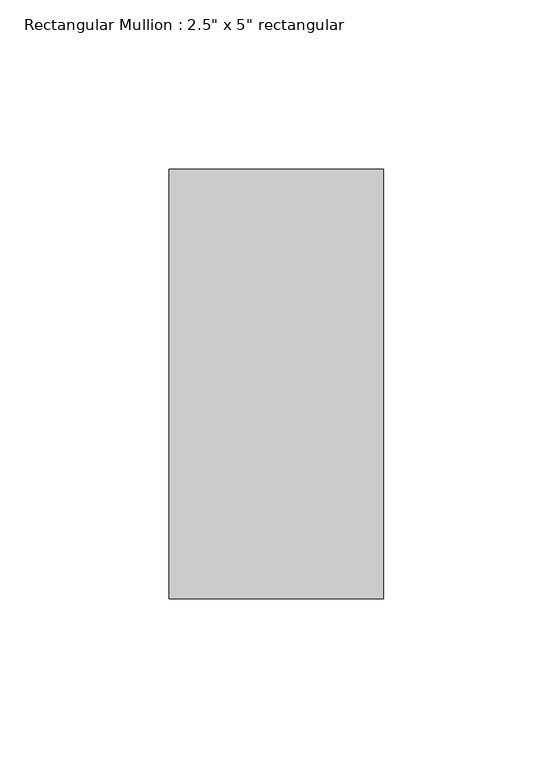
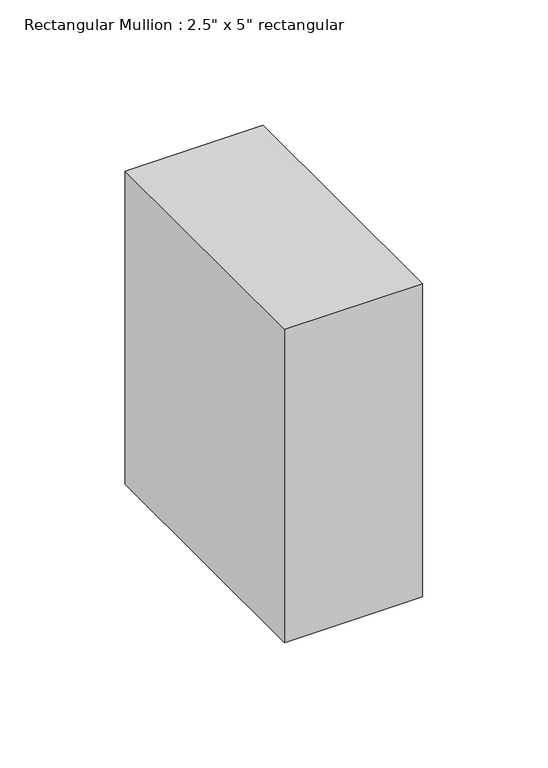
"""IFC4 building model written with IfcOpenShell, lengths in millimetres: member geometry."""

from ifc_helpers import new_model, si_unit, frame, origin, place, context, project, spatial, polyline, outline, extrude, source, transform, mapped, element, save


def member_f6f0dfdd(model_context):
    return source(origin(), model_context, "Body", "SweptSolid", [
        extrude(outline(polyline([(31.75, 63.5), (31.75, -63.5), (-31.75, -63.5), (-31.75, 63.5), (31.75, 63.5)])), frame((0.0, 0.0, -152.4), z_axis=(0.0, 0.0, 1.0), x_axis=(1.0, 0.0, 0.0)), (0.0, 0.0, 1.0), 152.4),
    ])


if __name__ == "__main__":
    model = new_model("IFC4")
    model_context = context("Model", 3, world=origin())
    ifc_project = project(units=[si_unit("LENGTHUNIT", "METRE", prefix="MILLI")], contexts=[model_context])
    site = spatial("IfcSite", under=ifc_project)
    building = spatial("IfcBuilding", under=site)
    placement = place(None, origin())
    member_shape = member_f6f0dfdd(model_context)
    element("IfcMember", 1, ObjectType="Rectangular Mullion : 2.5\" x 5\" rectangular", at=placement, inside=building, context=model_context, shape_type="MappedRepresentation", body=[
        mapped(member_shape, transform((0.0, 0.0, 0.0), x_axis=(1.0, 0.0, 0.0), y_axis=(0.0, 1.0, 0.0), z_axis=(0.0, 0.0, 1.0))),
    ])
    save(model, "model.ifc")

# Revit data of these elements
# Type "Rectangular Mullion : 2.5\" x 5\" rectangular"
#   built-in parameter 1007304 = 0.416667 (stored number, unit not read)
#   built-in parameter 1007301 = 0.104167 (stored number, unit not read)
#   built-in parameter 1007300 = 0.104167 (stored number, unit not read)
# Element 1 (IfcMember, "Rectangular Mullion : 2.5\" x 5\" rectangular")
#   Materials on its faces: "WINDOW FRAMING"
# Materials
#   "WINDOW FRAMING": class "Generic", colour RGB 120 120 120, transparency 0, Cost = 0
